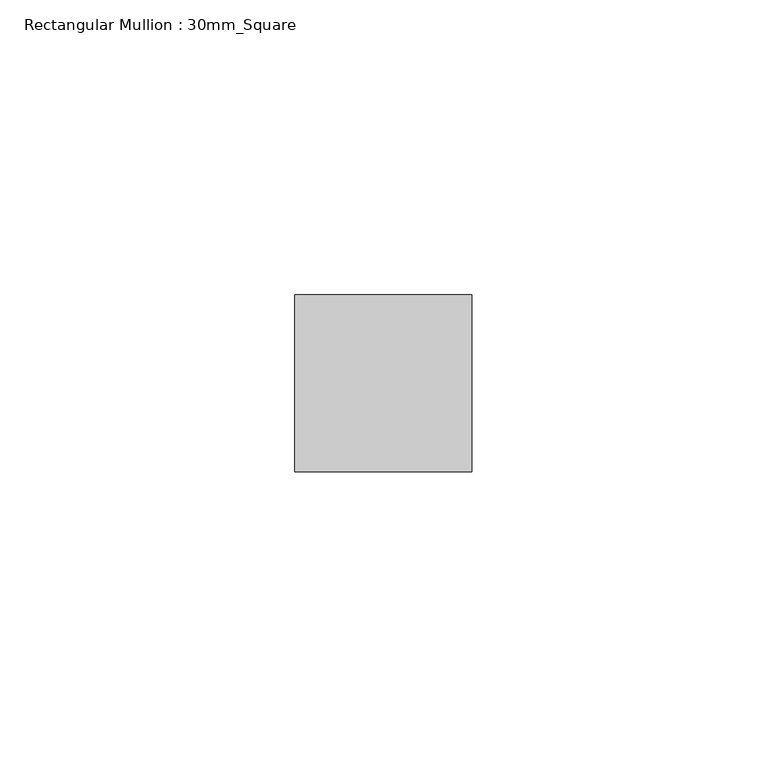
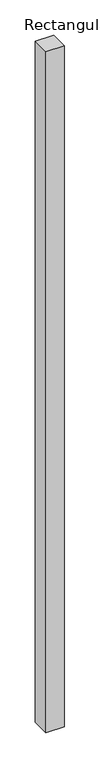
"""IFC4 building model written with IfcOpenShell, lengths in millimetres: member geometry, Rectangular Mullion : 30mm_Square."""

from ifc_helpers import new_model, si_unit, frame, origin, place, context, project, spatial, polyline, outline, extrude, source, transform, mapped, element, save


def rectangular_mullion_30mm_square_eb1e678b(model_context):
    return source(origin(), model_context, "Body", "SweptSolid", [
        extrude(outline(polyline([(0.0, 15.0), (0.0, -15.0), (-30.0, -15.0), (-30.0, 15.0), (0.0, 15.0)])), frame((0.0, 0.0, -1176.7008955), z_axis=(0.0, 0.0, 1.0), x_axis=(1.0, 0.0, 0.0)), (0.0, 0.0, 1.0), 1176.7008955),
    ])


if __name__ == "__main__":
    model = new_model("IFC4")
    model_context = context("Model", 3, world=origin())
    ifc_project = project(units=[si_unit("LENGTHUNIT", "METRE", prefix="MILLI")], contexts=[model_context])
    site = spatial("IfcSite", under=ifc_project)
    building = spatial("IfcBuilding", under=site)
    placement = place(None, origin())
    rectangular_mullion_30mm_square_shape = rectangular_mullion_30mm_square_eb1e678b(model_context)
    element("IfcMember", 1, ObjectType="Rectangular Mullion : 30mm_Square", at=placement, inside=building, context=model_context, shape_type="MappedRepresentation", body=[
        mapped(rectangular_mullion_30mm_square_shape, transform((0.0, 0.0, 0.0), x_axis=(1.0, 0.0, 0.0), y_axis=(0.0, 1.0, 0.0), z_axis=(0.0, 0.0, 1.0))),
    ])
    save(model, "model.ifc")

# Revit data of these elements
# Type "Rectangular Mullion : 30mm_Square"
#   Keynote = "H11"
#   built-in parameter 1007304 = 0.0984252 (stored number, unit not read)
#   built-in parameter 1007301 = 0.0492126 (stored number, unit not read)
#   built-in parameter 1007300 = 0.0492126 (stored number, unit not read)
# Element 1 (IfcMember, "Rectangular Mullion : 30mm_Square")
#   Materials on its faces: "Aluminium"
# Materials
#   "Aluminium": class "Metal", colour RGB 247 247 247, transparency 0, Description = "Aluminium 6061", Cost = 0
